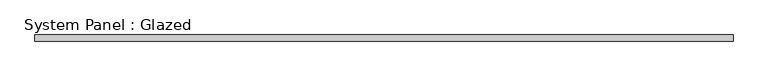
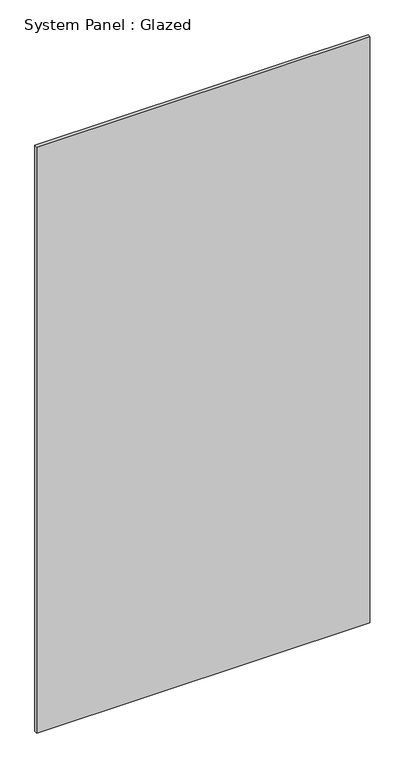
"""IFC4 building model written with IfcOpenShell, lengths in millimetres: plate geometry, System Panel : Glazed."""

from ifc_helpers import new_model, si_unit, origin, origin_with_axes, place, context, project, spatial, polyline, outline, extrude, source, transform, mapped, element, save


def system_panel_glazed_1ec048b2(model_context):
    return source(origin(), model_context, "Body", "SweptSolid", [
        extrude(outline(polyline([(1358.9, 19.05), (-1358.9, 19.05), (-1358.9, 44.45), (1358.9, 44.45), (1358.9, 19.05)])), origin_with_axes(), (0.0, 0.0, 1.0), 5054.6),
    ])


if __name__ == "__main__":
    model = new_model("IFC4")
    model_context = context("Model", 3, world=origin())
    ifc_project = project(units=[si_unit("LENGTHUNIT", "METRE", prefix="MILLI")], contexts=[model_context])
    site = spatial("IfcSite", under=ifc_project)
    building = spatial("IfcBuilding", under=site)
    placement = place(None, origin())
    system_panel_glazed_shape = system_panel_glazed_1ec048b2(model_context)
    element("IfcPlate", 1, ObjectType="System Panel : Glazed", at=placement, inside=building, context=model_context, shape_type="MappedRepresentation", body=[
        mapped(system_panel_glazed_shape, transform((0.0, 0.0, 0.0), x_axis=(1.0, 0.0, 0.0), y_axis=(0.0, 1.0, 0.0), z_axis=(0.0, 0.0, 1.0))),
    ])
    save(model, "model.ifc")

# Revit data of these elements
# Type "System Panel : Glazed"
#   Construction Type Id = "GSP4R"
#   Analytic Construction = "1/8 in Pilkington single glazing"
#   Visual Light Transmittance = 0.9
#   Solar Heat Gain Coefficient = 0.86
#   Heat Transfer Coefficient (U) = 1.18115 BTU/(h·ft²·°F)
# Element 1 (IfcPlate, "System Panel : Glazed")
#   Materials on its faces: "Glass"
# Materials
#   "Glass": class "Glass", colour RGB 0 128 192, transparency 0.75, Description = "Soda Lime Glass", Cost = 0
